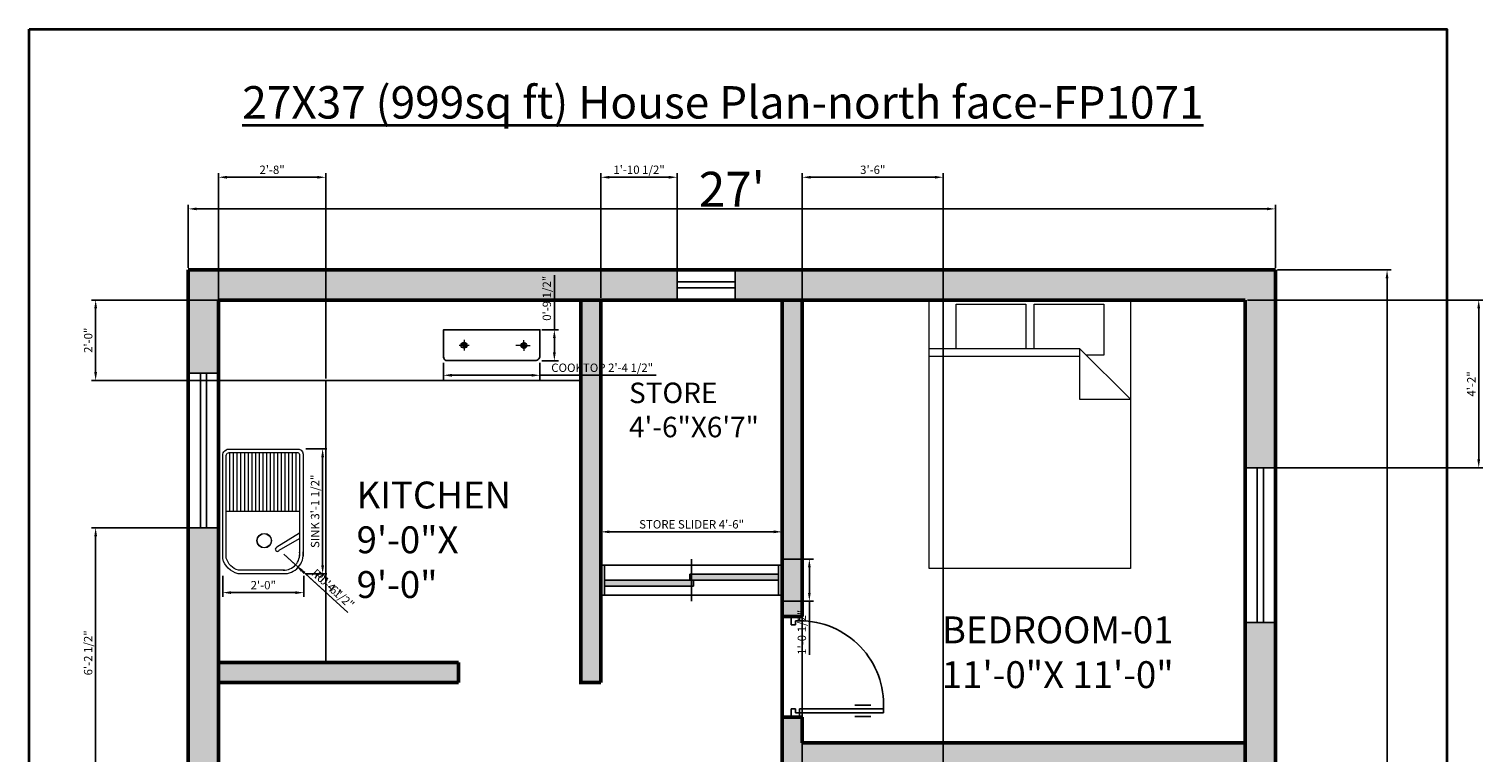
# Model space of a CAD drawing. Units: inches. Extents: x -36 to 398, y -51 to 516.
# Tile 3 of 3: x -36 to 398, y 300 to 516. Entities that reach past the tile are written whole.
import ezdxf

# ---------------------------------------------------------------- set-up
doc = ezdxf.new("R2010")
doc.units = ezdxf.units.IN
doc.header["$PDMODE"] = 34
for name, color, linetype, lineweight in [('A-ANNO-DIMS', 2, 'Continuous', 18), ('A-ANNO-TTLB', 7, 'Continuous', 35), ('A-AREA-IDEN', 7, 'Continuous', 25), ('A-DOOR', 170, 'Continuous', 25), ('A-EQPM', 8, 'Continuous', 18), ('A-FLOR-CASE', 7, 'Continuous', 25), ('A-FLOR-FIXT', 8, 'Continuous', 18), ('A-FURN', 8, 'Continuous', 18), ('A-GLAZ-PATT', 7, 'Continuous', 13), ('WALL', 7, 'Continuous', 50), ('WINDOW', 5, 'Continuous', 25)]:
    doc.layers.add(name, color=color, linetype=linetype, lineweight=lineweight)
doc.layers.add('A-WALL-PATT', color=251, linetype='Continuous', lineweight=13, true_color=0x636466)
doc.layers.add('dimensions', color=7, linetype='Continuous')
doc.styles.get("Standard").update_dxf_attribs({"font": 'arial.ttf'})
doc.dimstyles.new('ISO-25', dxfattribs={"dimtxt": 2.5, "dimasz": 2.5, "dimexe": 1.25, "dimexo": 0.625, "dimtad": 1, "dimdec": 1, "dimlunit": 3, "dimtxsty": 'Standard', "dimcen": 2.5, "dimadec": 0, "dimazin": 0, "dimtfac": 1, "dimtdec": 1, "dimtmove": 0, "dimatfit": 3, "dimfxl": 1, "dimarcsym": 0})

# ---------------------------------------------------------------- blocks, each defined once
blk = doc.blocks.new('WD_00_X1')
for p, q in [((-0.5, 0.5), (0.5, 0.5)), ((-0.48, 0.5), (-0.48, -0.5)), ((0.48, 0.5), (0.48, -0.5)), ((0.48, 0.1), (-0.48, 0.1)), ((0.48, -0.1), (-0.48, -0.1)), ((-0.5, -0.5), (0.5, -0.5))]:
    blk.add_line(p, q)
blk = doc.blocks.new('DR_UKF1')
for p, q in [((-0.458, 0.042), (-0.458, 0.875)), ((-0.458, 0.875), (-0.417, 0.875)), ((-0.417, 0.875), (-0.417, 0.042)), ((-0.494, 0.751), (-0.494, 0.59)), ((-0.381, 0.751), (-0.381, 0.59)), ((-0.5, -0.042), (-0.5, 0.042)), ((-0.5, 0.042), (-0.458, 0.042)), ((-0.417, 0.042), (-0.458, 0.042)), ((-0.458, 0.042), (-0.458, 0)), ((-0.458, 0), (-0.417, 0)), ((-0.417, 0), (-0.417, -0.042)), ((0.417, 0), (0.417, -0.042)), ((0.458, 0), (0.417, 0)), ((0.458, 0.042), (0.458, 0)), ((0.5, 0.042), (0.458, 0.042)), ((0.5, -0.042), (0.5, 0.042)), ((-0.417, -0.042), (-0.5, -0.042)), ((-0.5, -0.042), (-0.5, -0.042)), ((0.417, -0.042), (0.5, -0.042)), ((0.5, -0.042), (0.5, -0.042))]:
    blk.add_line(p, q)
blk.add_arc((-0.375, 0.043), 0.833, 359.9283, 92.866)
blk = doc.blocks.new('SINK')
for p, q in [((2.41, 0.46), (2.41, -20.67)), ((3.73, 0.46), (3.73, -20.67)), ((5.05, 0.46), (5.05, -20.67)), ((6.38, 0.46), (6.38, -20.67)), ((7.7, 0.46), (7.7, -20.67)), ((9.03, 0.46), (9.03, -20.67)), ((10.35, 0.46), (10.35, -20.67)), ((11.67, 0.46), (11.67, -20.67)), ((13, 0.46), (13, -20.67)), ((14.32, 0.46), (14.32, -20.67)), ((15.64, 0.46), (15.64, -20.67)), ((16.97, 0.46), (16.97, -20.67)), ((18.29, 0.46), (18.29, -20.67)), ((19.62, 0.46), (19.62, -20.67)), ((20.94, 0.46), (20.94, -20.67)), ((22.26, 0.46), (22.26, -20.67)), ((23.59, 0.46), (23.59, -20.67)), ((24.91, 0.46), (24.91, -20.67)), ((26.24, 0.46), (26.24, -20.67)), ((1.2, -20.67), (27.56, -20.67)), ((27.56, -28.49), (19.38, -33.59)), ((20.23, -34.64), (27.56, -30.49))]:
    blk.add_line(p, q)
for points in [[(22.1, -43.09), (5.43, -43.09, -0.278946), (-0.08, -37.68), (-0.08, -0.62, -0.442838), (2.54, 1.74, -0.442838)], [(22.1, -41.81), (5.59, -41.81, -0.266071), (1.2, -37.51), (1.2, -0.62, -0.442099), (2.41, 0.46)], [(2.18, 1.74), (26.61, 1.74, -0.390462), (28.84, -0.06), (28.84, -20.67)], [(2.18, 0.46), (26.66, 0.46, -0.376515), (27.56, -0.18), (27.56, -20.67)]]:
    blk.add_lwpolyline(points, format="xyb")
for points in [[(27.56, -0.18), (27.56, -36.84)], [(28.84, -0.18), (28.84, -36.84)]]:
    blk.add_lwpolyline(points)
for radius in [2.63, 2.53]:
    blk.add_circle((14.84, -31.22), radius)
for centre, radius, start, end in [((19.56, -34.32), 0.748, 103.6237, 334.3933), ((21.9, -36.1), 6.99, 267.9726, 7.4622), ((21.9, -36.1), 5.71, 267.9726, 7.4622)]:
    blk.add_arc(centre, radius, start, end)
blk = doc.blocks.new('WD_00_X2')
for p, q in [((0, 0.7), (0, -0.7)), ((-0.5, 0.5), (0.5, 0.5)), ((-0.48, 0.5), (-0.48, -0.5)), ((0.48, 0.5), (0.48, -0.5)), ((0.01, 0.2), (-0.48, 0.2)), ((0.01, 0.2), (0.01, 0)), ((0.48, 0), (-0.48, 0)), ((-0.01, 0), (-0.01, -0.2)), ((0.48, -0.2), (-0.01, -0.2)), ((-0.5, -0.5), (0.5, -0.5))]:
    blk.add_line(p, q)
blk = doc.blocks.new('GAS STOVE')
at = {"layer": 'dimensions'}
for points in [[(0.01, -8.39), (0, -8.07), (0, 0), (28.69, 0), (28.69, -7.85)], [(26.99, -9.22), (0.89, -9.22)]]:
    blk.add_lwpolyline(points, dxfattribs=at)
for centre, radius, start, end in [((0.99, -8.22), 1, 171.6035, 275.6391), ((27.21, -7.75), 1.48, 261.2373, 356.1184)]:
    blk.add_arc(centre, radius, start, end, dxfattribs=at)
for p in [(6.09, -4.63), (23.92, -4.73)]:
    blk.add_point(p, dxfattribs=at)
blk = doc.blocks.new('new block')
for p, q in [((6.13, -3.04), (6.13, -6.22)), ((23.92, -4.73), (23.92, -3.08)), ((4.65, -4.66), (7.63, -4.66)), ((23.92, -4.73), (21.5, -4.73)), ((23.92, -4.73), (25.8, -4.73)), ((23.92, -4.73), (23.92, -6.28))]:
    blk.add_line(p, q)
for centre, radius in [((6.09, -4.63), 0.897), ((23.92, -4.73), 0.857)]:
    blk.add_circle(centre, radius)
blk.add_blockref('GAS STOVE', (0, 0))
blk = doc.blocks.new('Bed - Queen')
for p, q in [((0, -80.00003), (0, 0)), ((0, 0), (59.99999, 0)), ((59.99999, 0), (59.99999, -80.00003)), ((7.99999, -1.2), (28.79998, -1.2)), ((7.99999, -14.4), (7.99999, -1.2)), ((28.79998, -1.2), (28.79998, -14.4)), ((31.19999, -1.2), (51.99999, -1.2)), ((31.19999, -14.4), (31.19999, -1.2)), ((51.99999, -1.2), (51.99999, -16.4)), ((0, -14.4), (44.8, -14.4)), ((44.8, -16.8), (0, -16.8)), ((59.99999, -29.6), (44.8, -14.4)), ((44.8, -14.4), (44.8, -29.6)), ((51.99999, -16.4), (46.79936, -16.4)), ((44.8, -29.6), (59.99999, -29.6)), ((59.99999, -80.00003), (0, -80.00003))]:
    blk.add_line(p, q)
blk = doc.blocks.new('*D15')
at = {"layer": 'A-ANNO-DIMS', "color": 0, "lineweight": -2, "transparency": 16777216}
for p, q in [((11.71, 444.6), (11.71, 463.4)), ((14.21, 462.15), (333.21, 462.15)), ((335.71, 444.6), (335.71, 463.4))]:
    blk.add_line(p, q, dxfattribs=at)
at = {"layer": 'A-ANNO-DIMS', "color": 0, "transparency": 16777216}
for points in [[(14.21, 462.57), (14.21, 461.73), (11.71, 462.15)], [(333.21, 462.57), (333.21, 461.73), (335.71, 462.15)]]:
    blk.add_solid(points, dxfattribs=at)
at = {"layer": 'Defpoints', "color": 0, "transparency": 16777216}
for p in [(335.71, 462.15), (11.71, 443.98), (335.71, 443.98)]:
    blk.add_point(p, dxfattribs=at)
at = {"layer": 'A-ANNO-DIMS', "color": 0, "transparency": 16777216, "insert": (173.71, 468), "char_height": 2.5, "attachment_point": 5}
blk.add_mtext("{\\H4.16x;27'}", dxfattribs=at)
blk = doc.blocks.new('*D16')
at = {"layer": 'A-ANNO-DIMS', "color": 0, "lineweight": -2, "transparency": 16777216}
for p, q in [((336.34, 443.98), (370.23, 443.98)), ((368.98, 441.48), (368.98, 2.48)), ((336.34, -0.02), (370.23, -0.02))]:
    blk.add_line(p, q, dxfattribs=at)
at = {"layer": 'A-ANNO-DIMS', "color": 0, "transparency": 16777216}
for points in [[(368.56, 441.48), (369.39, 441.48), (368.98, 443.98)], [(368.56, 2.48), (369.39, 2.48), (368.98, -0.02)]]:
    blk.add_solid(points, dxfattribs=at)
at = {"layer": 'Defpoints', "color": 0, "transparency": 16777216}
for p in [(335.71, 443.98), (335.71, -0.02), (368.98, -0.02)]:
    blk.add_point(p, dxfattribs=at)
at = {"layer": 'A-ANNO-DIMS', "color": 0, "transparency": 16777216, "insert": (363.04, 221.98), "char_height": 2.5, "attachment_point": 5, "rotation": 90}
blk.add_mtext("{\\H4.16x;37'}", dxfattribs=at)
blk = doc.blocks.new('*D28')
at = {"layer": 'A-ANNO-DIMS', "color": 0, "lineweight": -2, "transparency": 16777216}
for p, q in [((46.79, 390.64), (53, 390.64)), ((51.75, 355.86), (51.75, 388.14)), ((46.79, 353.36), (53, 353.36))]:
    blk.add_line(p, q, dxfattribs=at)
at = {"layer": 'A-ANNO-DIMS', "color": 0, "transparency": 16777216}
for points in [[(51.34, 388.14), (52.17, 388.14), (51.75, 390.64)], [(51.34, 355.86), (52.17, 355.86), (51.75, 353.36)]]:
    blk.add_solid(points, dxfattribs=at)
at = {"layer": 'Defpoints', "color": 0, "transparency": 16777216}
for p in [(46.16, 390.64), (51.75, 390.64), (46.16, 353.36)]:
    blk.add_point(p, dxfattribs=at)
at = {"layer": 'A-ANNO-DIMS', "color": 0, "transparency": 16777216, "insert": (49.83, 372), "char_height": 2.5, "attachment_point": 5, "rotation": 90}
blk.add_mtext('SINK 3\'-1 1/2"', dxfattribs=at)
blk = doc.blocks.new('*D29')
at = {"layer": 'A-ANNO-DIMS', "color": 0, "lineweight": -2, "transparency": 16777216}
for p, q in [((21.97, 352.73), (21.97, 346.51)), ((46.16, 352.73), (46.16, 346.51)), ((24.47, 347.76), (43.66, 347.76))]:
    blk.add_line(p, q, dxfattribs=at)
at = {"layer": 'A-ANNO-DIMS', "color": 0, "transparency": 16777216}
for points in [[(24.47, 348.18), (24.47, 347.35), (21.97, 347.76)], [(43.66, 348.18), (43.66, 347.35), (46.16, 347.76)]]:
    blk.add_solid(points, dxfattribs=at)
at = {"layer": 'Defpoints', "color": 0, "transparency": 16777216}
for p in [(21.97, 353.36), (46.16, 353.36), (46.16, 347.76)]:
    blk.add_point(p, dxfattribs=at)
at = {"layer": 'A-ANNO-DIMS', "color": 0, "transparency": 16777216, "insert": (34.07, 349.66), "char_height": 2.5, "attachment_point": 5}
blk.add_mtext('2\'-0"', dxfattribs=at)
blk = doc.blocks.new('*D30')
at = {"layer": 'A-ANNO-DIMS', "color": 0, "lineweight": -2, "transparency": 16777216}
for p, q in [((134.71, 358.41), (134.71, 367.13)), ((137.21, 365.88), (186.21, 365.88)), ((188.71, 358.41), (188.71, 367.13))]:
    blk.add_line(p, q, dxfattribs=at)
at = {"layer": 'A-ANNO-DIMS', "color": 0, "transparency": 16777216}
for points in [[(137.21, 366.3), (137.21, 365.47), (134.71, 365.88)], [(186.21, 366.3), (186.21, 365.47), (188.71, 365.88)]]:
    blk.add_solid(points, dxfattribs=at)
at = {"layer": 'Defpoints', "color": 0, "transparency": 16777216}
for p in [(188.71, 365.88), (134.71, 357.78), (188.71, 357.78)]:
    blk.add_point(p, dxfattribs=at)
at = {"layer": 'A-ANNO-DIMS', "color": 0, "transparency": 16777216, "insert": (161.71, 367.8), "char_height": 2.5, "attachment_point": 5}
blk.add_mtext('STORE SLIDER 4\'-6"', dxfattribs=at)
blk = doc.blocks.new('*D31')
at = {"layer": 'A-ANNO-DIMS', "color": 0, "lineweight": -2, "transparency": 16777216}
for p, q in [((189.34, 357.78), (198.06, 357.78)), ((196.81, 355.28), (196.81, 347.68)), ((189.34, 345.18), (198.06, 345.18)), ((196.81, 345.18), (196.81, 329.2))]:
    blk.add_line(p, q, dxfattribs=at)
at = {"layer": 'A-ANNO-DIMS', "color": 0, "transparency": 16777216}
for points in [[(196.4, 355.28), (197.23, 355.28), (196.81, 357.78)], [(196.4, 347.68), (197.23, 347.68), (196.81, 345.18)]]:
    blk.add_solid(points, dxfattribs=at)
at = {"layer": 'Defpoints', "color": 0, "transparency": 16777216}
for p in [(188.71, 357.78), (188.71, 345.18), (196.81, 345.18)]:
    blk.add_point(p, dxfattribs=at)
at = {"layer": 'A-ANNO-DIMS', "color": 0, "transparency": 16777216, "insert": (194.9, 335.94), "char_height": 2.5, "attachment_point": 5, "rotation": 90}
blk.add_mtext('1\'-0 1/2"', dxfattribs=at)
blk = doc.blocks.new('*D32')
at = {"layer": 'A-ANNO-DIMS', "color": 0, "lineweight": -2, "transparency": 16777216}
for p, q in [((87.77, 416.23), (87.77, 411.3)), ((116.51, 416.23), (116.51, 411.3)), ((90.27, 412.55), (114.01, 412.55)), ((116.51, 412.55), (151.13, 412.55))]:
    blk.add_line(p, q, dxfattribs=at)
at = {"layer": 'A-ANNO-DIMS', "color": 0, "transparency": 16777216}
for points in [[(90.27, 412.97), (90.27, 412.13), (87.77, 412.55)], [(114.01, 412.97), (114.01, 412.13), (116.51, 412.55)]]:
    blk.add_solid(points, dxfattribs=at)
at = {"layer": 'Defpoints', "color": 0, "transparency": 16777216}
for p in [(87.77, 416.86), (116.51, 416.86), (116.51, 412.55)]:
    blk.add_point(p, dxfattribs=at)
at = {"layer": 'A-ANNO-DIMS', "color": 0, "transparency": 16777216, "insert": (135.07, 414.47), "char_height": 2.5, "attachment_point": 5}
blk.add_mtext('COOKTOP 2\'-4 1/2"', dxfattribs=at)
blk = doc.blocks.new('*D33')
at = {"layer": 'A-ANNO-DIMS', "color": 0, "lineweight": -2, "transparency": 16777216}
for p, q in [((120.82, 426.14), (120.82, 442.36)), ((117.13, 426.14), (122.07, 426.14)), ((120.82, 419.36), (120.82, 423.64)), ((117.13, 416.86), (122.07, 416.86))]:
    blk.add_line(p, q, dxfattribs=at)
at = {"layer": 'A-ANNO-DIMS', "color": 0, "transparency": 16777216}
for points in [[(120.4, 423.64), (121.23, 423.64), (120.82, 426.14)], [(120.4, 419.36), (121.23, 419.36), (120.82, 416.86)]]:
    blk.add_solid(points, dxfattribs=at)
at = {"layer": 'Defpoints', "color": 0, "transparency": 16777216}
for p in [(116.51, 426.14), (120.82, 426.14), (116.51, 416.86)]:
    blk.add_point(p, dxfattribs=at)
at = {"layer": 'A-ANNO-DIMS', "color": 0, "transparency": 16777216, "insert": (118.9, 435.5), "char_height": 2.5, "attachment_point": 5, "rotation": 90}
blk.add_mtext('0\'-9 1/2"', dxfattribs=at)
blk = doc.blocks.new('*D39')
at = {"layer": 'A-ANNO-DIMS', "color": 0, "lineweight": -2, "transparency": 16777216}
for p, q in [((11.09, 367.07), (-17.14, 367.07)), ((-15.89, 295.04), (-15.89, 364.57)), ((11.09, 292.54), (-17.14, 292.54))]:
    blk.add_line(p, q, dxfattribs=at)
at = {"layer": 'A-ANNO-DIMS', "color": 0, "transparency": 16777216}
for points in [[(-16.3, 364.57), (-15.47, 364.57), (-15.89, 367.07)], [(-16.3, 295.04), (-15.47, 295.04), (-15.89, 292.54)]]:
    blk.add_solid(points, dxfattribs=at)
at = {"layer": 'Defpoints', "color": 0, "transparency": 16777216}
for p in [(-15.89, 367.07), (11.71, 367.07), (11.71, 292.54)]:
    blk.add_point(p, dxfattribs=at)
at = {"layer": 'A-ANNO-DIMS', "color": 0, "transparency": 16777216, "insert": (-17.8, 329.81), "char_height": 2.5, "attachment_point": 5, "rotation": 90}
blk.add_mtext('6\'-2 1/2"', dxfattribs=at)
blk = doc.blocks.new('*D40')
at = {"layer": 'A-ANNO-DIMS', "color": 0, "lineweight": -2, "transparency": 16777216}
for p, q in [((134.71, 435.6), (134.71, 472.83)), ((157.41, 435.6), (157.41, 472.83)), ((137.21, 471.58), (154.91, 471.58))]:
    blk.add_line(p, q, dxfattribs=at)
at = {"layer": 'A-ANNO-DIMS', "color": 0, "transparency": 16777216}
for points in [[(137.21, 471.99), (137.21, 471.16), (134.71, 471.58)], [(154.91, 471.99), (154.91, 471.16), (157.41, 471.58)]]:
    blk.add_solid(points, dxfattribs=at)
at = {"layer": 'Defpoints', "color": 0, "transparency": 16777216}
for p in [(157.41, 471.58), (134.71, 434.98), (157.41, 434.98)]:
    blk.add_point(p, dxfattribs=at)
at = {"layer": 'A-ANNO-DIMS', "color": 0, "transparency": 16777216, "insert": (146.06, 473.49), "char_height": 2.5, "attachment_point": 5}
blk.add_mtext('1\'-10 1/2"', dxfattribs=at)
blk = doc.blocks.new('*D41')
at = {"layer": 'A-ANNO-DIMS', "color": 0, "lineweight": -2, "transparency": 16777216}
for p, q in [((327.34, 434.98), (397.55, 434.98)), ((396.3, 432.48), (396.3, 387.47)), ((327.34, 384.97), (397.55, 384.97))]:
    blk.add_line(p, q, dxfattribs=at)
at = {"layer": 'A-ANNO-DIMS', "color": 0, "transparency": 16777216}
for points in [[(395.88, 432.48), (396.71, 432.48), (396.3, 434.98)], [(395.88, 387.47), (396.71, 387.47), (396.3, 384.97)]]:
    blk.add_solid(points, dxfattribs=at)
at = {"layer": 'Defpoints', "color": 0, "transparency": 16777216}
for p in [(326.71, 434.98), (326.71, 384.97), (396.3, 384.97)]:
    blk.add_point(p, dxfattribs=at)
at = {"layer": 'A-ANNO-DIMS', "color": 0, "transparency": 16777216, "insert": (394.42, 409.97), "char_height": 2.5, "attachment_point": 5, "rotation": 90}
blk.add_mtext('4\'-2"', dxfattribs=at)
blk = doc.blocks.new('*D45')
at = {"layer": 'A-ANNO-DIMS', "color": 0, "lineweight": -2, "transparency": 16777216}
for p, q in [((20.71, 413.78), (20.71, 472.83)), ((52.67, 411.6), (52.67, 472.83)), ((23.21, 471.58), (50.17, 471.58))]:
    blk.add_line(p, q, dxfattribs=at)
at = {"layer": 'A-ANNO-DIMS', "color": 0, "transparency": 16777216}
for points in [[(23.21, 471.99), (23.21, 471.16), (20.71, 471.58)], [(50.17, 471.99), (50.17, 471.16), (52.67, 471.58)]]:
    blk.add_solid(points, dxfattribs=at)
at = {"layer": 'Defpoints', "color": 0, "transparency": 16777216}
for p in [(52.67, 471.58), (20.71, 413.15), (52.67, 410.98)]:
    blk.add_point(p, dxfattribs=at)
at = {"layer": 'A-ANNO-DIMS', "color": 0, "transparency": 16777216, "insert": (36.69, 473.48), "char_height": 2.5, "attachment_point": 5}
blk.add_mtext('2\'-8"', dxfattribs=at)
blk = doc.blocks.new('*D46')
at = {"layer": 'A-ANNO-DIMS', "color": 0, "lineweight": -2, "transparency": 16777216}
for p, q in [((128.09, 434.98), (-17.14, 434.98)), ((-15.89, 413.48), (-15.89, 432.48)), ((128.09, 410.98), (-17.14, 410.98))]:
    blk.add_line(p, q, dxfattribs=at)
at = {"layer": 'A-ANNO-DIMS', "color": 0, "transparency": 16777216}
for points in [[(-16.3, 432.48), (-15.47, 432.48), (-15.89, 434.98)], [(-16.3, 413.48), (-15.47, 413.48), (-15.89, 410.98)]]:
    blk.add_solid(points, dxfattribs=at)
at = {"layer": 'Defpoints', "color": 0, "transparency": 16777216}
for p in [(-15.89, 434.98), (128.71, 434.98), (128.71, 410.98)]:
    blk.add_point(p, dxfattribs=at)
at = {"layer": 'A-ANNO-DIMS', "color": 0, "transparency": 16777216, "insert": (-17.79, 422.98), "char_height": 2.5, "attachment_point": 5, "rotation": 90}
blk.add_mtext('2\'-0"', dxfattribs=at)
blk = doc.blocks.new('*D50')
at = {"layer": 'A-ANNO-DIMS', "color": 0, "lineweight": -2, "transparency": 16777216}
for p, q in [((194.71, 248.83), (194.71, 472.83)), ((236.71, 277.21), (236.71, 472.83)), ((197.21, 471.58), (234.21, 471.58))]:
    blk.add_line(p, q, dxfattribs=at)
at = {"layer": 'A-ANNO-DIMS', "color": 0, "transparency": 16777216}
for points in [[(197.21, 471.99), (197.21, 471.16), (194.71, 471.58)], [(234.21, 471.99), (234.21, 471.16), (236.71, 471.58)]]:
    blk.add_solid(points, dxfattribs=at)
at = {"layer": 'Defpoints', "color": 0, "transparency": 16777216}
for p in [(236.71, 471.58), (236.71, 276.58), (194.71, 248.21)]:
    blk.add_point(p, dxfattribs=at)
at = {"layer": 'A-ANNO-DIMS', "color": 0, "transparency": 16777216, "insert": (215.71, 473.48), "char_height": 2.5, "attachment_point": 5}
blk.add_mtext('3\'-6"', dxfattribs=at)
blk = doc.blocks.new('*D53')
at = {"layer": 'A-ANNO-DIMS', "color": 0, "lineweight": -2, "transparency": 16777216}
for p, q in [((40.19, 359.21), (44.48, 355.31)), ((55.79, 345.02), (46.33, 353.63))]:
    blk.add_line(p, q, dxfattribs=at)
at = {"layer": 'A-ANNO-DIMS', "color": 0, "transparency": 16777216}
blk.add_solid([(46.61, 353.94), (46.05, 353.32), (44.48, 355.31)], dxfattribs=at)
at = {"layer": 'Defpoints', "color": 0, "transparency": 16777216}
for p in [(40.19, 359.21), (44.48, 355.31)]:
    blk.add_point(p, dxfattribs=at)
at = {"layer": 'A-ANNO-DIMS', "color": 0, "transparency": 16777216, "insert": (53.26, 349.89), "char_height": 2.5, "attachment_point": 5, "rotation": 317.7157}
blk.add_mtext('R0\'-6"', dxfattribs=at)
blk = doc.blocks.new('*D54')
at = {"layer": 'A-ANNO-DIMS', "color": 0, "lineweight": -2, "transparency": 16777216}
for p, q in [((40.19, 359.21), (43.69, 356.02)), ((59.31, 341.82), (45.54, 354.34))]:
    blk.add_line(p, q, dxfattribs=at)
at = {"layer": 'A-ANNO-DIMS', "color": 0, "transparency": 16777216}
blk.add_solid([(45.82, 354.65), (45.26, 354.03), (43.69, 356.02)], dxfattribs=at)
at = {"layer": 'Defpoints', "color": 0, "transparency": 16777216}
for p in [(40.19, 359.21), (43.69, 356.02)]:
    blk.add_point(p, dxfattribs=at)
at = {"layer": 'A-ANNO-DIMS', "color": 0, "transparency": 16777216, "insert": (54.64, 348.66), "char_height": 2.5, "attachment_point": 5, "rotation": 317.7166}
blk.add_mtext('R0\'-4 1/2"', dxfattribs=at)

msp = doc.modelspace()

# ---------------------------------------------------------------- hatches: boundary and pattern name
at = {"layer": 'A-GLAZ-PATT'}
h = msp.add_hatch(color=256, dxfattribs=at)
h.dxf.hatch_style = 1
h.paths.add_polyline_path([(187.63, 351.48), (187.63, 353.28), (161.71, 353.28), (161.71, 351.48)])
h.paths.add_polyline_path([(135.79, 351.48), (135.79, 349.68), (161.71, 349.68), (161.71, 351.48)])
at = {"layer": 'A-WALL-PATT'}
h = msp.add_hatch(color=256, dxfattribs=at)
h.dxf.hatch_style = 1
h.paths.add_polyline_path([(335.71, 155.4), (326.71, 155.4), (326.71, 154.44), (326.71, 50.65), (335.71, 50.65), (335.71, 51.01)])
h.paths.add_polyline_path([(335.71, 257.33), (326.71, 257.33), (326.71, 256.97), (326.71, 201.48), (335.71, 201.48), (335.71, 202.44)])
h.paths.add_polyline_path([(335.71, 33.37), (326.71, 33.37), (326.71, 33.01), (326.71, 8.98), (200.71, 8.98), (148.47, 8.98), (148.47, -0.02), (335.71, -0.02)])
h.paths.add_polyline_path([(118.44, 5.24), (118.46, 8.98), (92.19, 8.98), (92.19, -0.02), (93.15, -0.02), (118.46, -0.02), (118.46, 2.74), (118.44, 2.74)])
h.paths.add_polyline_path([(20.71, 85.44), (11.71, 85.44), (11.71, 84.48), (11.71, -0.02), (46.11, -0.02), (46.11, 8.98), (45.15, 8.98), (20.71, 8.98)])
h.paths.add_polyline_path([(20.71, 246.46), (11.71, 246.46), (11.71, 245.5), (11.71, 131.52), (20.71, 131.52), (20.71, 132.48)])
h.paths.add_polyline_path([(152.93, 182.98), (20.71, 182.98), (20.71, 176.98), (152.93, 176.98)])
h.paths.add_polyline_path([(188.71, 182.98), (182.93, 182.98), (182.93, 176.98), (188.71, 176.98)])
h.paths.add_polyline_path([(194.71, 224.98), (199.29, 224.98), (199.29, 230.98), (188.71, 230.98), (188.71, 79.98), (210.71, 79.98), (210.71, 80.98), (326.71, 80.98), (326.71, 85.98), (194.71, 85.98)])
h.paths.add_polyline_path([(326.71, 230.98), (229.41, 230.98), (229.41, 224.98), (326.71, 224.98)], flags=0)
h.paths.add_polyline_path([(242.71, 276.58), (236.71, 276.58), (236.71, 230.98), (242.71, 230.98)])
h.paths.add_polyline_path([(326.71, 302.98), (194.71, 302.98), (194.71, 310.64), (188.71, 310.64), (188.71, 296.98), (326.71, 296.98)])
h.paths.add_polyline_path([(242.71, 296.98), (236.71, 296.98), (236.71, 294.58), (242.71, 294.58)])
h.paths.add_polyline_path([(194.71, 434.98), (188.71, 434.98), (188.71, 340.61), (191.4, 340.61), (191.4, 340.64), (193.9, 340.64), (194.71, 340.61)])
h.paths.add_polyline_path([(335.71, 443.98), (174.69, 443.98), (174.69, 434.98), (175.05, 434.98), (326.71, 434.98), (326.71, 384.97), (335.71, 384.97), (335.71, 385.93)])
h.paths.add_polyline_path([(335.71, 338.89), (326.71, 338.89), (326.71, 337.93), (326.71, 274.61), (335.71, 274.61), (335.71, 274.97)])
h.paths.add_polyline_path([(157.41, 443.98), (157.05, 443.98), (11.71, 443.98), (11.71, 413.15), (20.71, 413.15), (20.71, 414.11), (20.71, 434.98), (157.41, 434.98)])
h.paths.add_polyline_path([(20.71, 367.07), (11.71, 367.07), (11.71, 366.11), (11.71, 292.54), (20.71, 292.54), (20.71, 293.5)])
h = msp.add_hatch(color=256, dxfattribs=at)
h.dxf.hatch_style = 1
h.paths.add_polyline_path([(20.71, 326.98), (20.71, 320.98), (92.29, 320.98), (92.29, 326.98)])
h.paths.add_polyline_path([(128.71, 320.98), (134.71, 320.98), (134.71, 434.98), (128.71, 434.98)])

# ---------------------------------------------------------------- linework, layer by layer
at = {"layer": 'A-ANNO-TTLB'}
msp.add_lwpolyline([(-35.73, 515.75), (386.76, 515.75), (386.76, -51.27), (-35.73, -51.27)], close=True, dxfattribs=at)
at = {"layer": 'A-FLOR-CASE'}
for p, q in [((128.71, 410.98), (52.67, 410.98)), ((52.67, 410.98), (52.67, 326.98))]:
    msp.add_line(p, q, dxfattribs=at)
at = {"layer": 'WALL'}
for p, q in [((11.71, -0.02), (11.71, 443.98)), ((11.71, 443.98), (335.71, 443.98)), ((335.71, -0.02), (335.71, 443.98)), ((20.71, 434.98), (326.71, 434.98)), ((20.71, 434.98), (20.71, 8.98)), ((128.71, 320.98), (128.71, 434.98)), ((134.71, 320.98), (134.71, 434.98)), ((188.71, 296.98), (188.71, 434.98)), ((194.71, 340.61), (194.71, 434.98)), ((326.71, 8.98), (326.71, 434.98)), ((194.71, 340.61), (188.71, 340.61)), ((20.71, 326.98), (92.29, 326.98)), ((92.29, 320.98), (92.29, 326.98)), ((20.71, 320.98), (92.29, 320.98)), ((128.21, 320.98), (134.71, 320.98)), ((188.71, 310.64), (194.71, 310.64)), ((194.71, 302.98), (194.71, 310.64)), ((194.71, 302.98), (326.71, 302.98))]:
    msp.add_line(p, q, dxfattribs=at)

# ---------------------------------------------------------------- block references
at = {"layer": 'A-DOOR', "xscale": -30, "yscale": 30, "zscale": 30, "rotation": 270.0000000000237}
msp.add_blockref('DR_UKF1', (192.65, 325.64), dxfattribs=at)
at = {"layer": 'A-EQPM'}
msp.add_blockref('new block', (87.82, 426.14), dxfattribs=at)
at = {"layer": 'A-FLOR-FIXT', "xscale": 0.8289137605783039, "yscale": 0.8289137605783039, "zscale": 0.8289137605783039}
msp.add_blockref('SINK', (22.04, 389.13), dxfattribs=at)
at = {"layer": 'A-FURN'}
msp.add_blockref('Bed - Queen', (232.56, 434.98), dxfattribs=at)
at = {"layer": 'WINDOW', "xscale": 18, "yscale": 9, "zscale": 18}
msp.add_blockref('WD_00_X1', (166.05, 439.48), dxfattribs=at)
at = {"layer": 'WINDOW', "yscale": 9}
for name, p, xscale, zscale, rotation in [('WD_00_X1', (16.21, 390.11), 48, 48, 89.99999999999999), ('WD_00_X1', (331.21, 361.93), 48, 48, 89.99999999999999), ('WD_00_X2', (161.71, 351.48), -54, 54, 180)]:
    msp.add_blockref(name, p, dxfattribs=dict(at, xscale=xscale, zscale=zscale, rotation=rotation))

# ---------------------------------------------------------------- texts
at = {"layer": 'A-ANNO-TTLB', "insert": (27.79, 498.74), "char_height": 9.6617, "attachment_point": 1}
msp.add_mtext_dynamic_manual_height_columns('{\\fArial|b1|i0|c0|p34;\\L27X37 (999sq ft) House Plan-north face-FP1071}', width=305.8474, gutter_width=48.31, heights=[0], dxfattribs=at)
at = {"layer": 'A-AREA-IDEN', "attachment_point": 1}
for s, width, gutter_width, insert, char_height in [('STORE \\P4\'-6"X6\'7"', 43.6398, 30.54, (143.07, 410.36), 6.108), ('KITCHEN\\P9\'-0"X 9\'-0"', 56.1888, 40.03, (61.87, 380.86), 8.0065), ('BEDROOM-01\\P11\'-0"X 11\'-0"', 96.1834, 40.03, (236.29, 340.66), 8.0065)]:
    msp.add_mtext_dynamic_manual_height_columns(s, width=width, gutter_width=gutter_width, heights=[0], dxfattribs=dict(at, insert=insert, char_height=char_height))

# ---------------------------------------------------------------- dimensions: what is measured, and where the dimension line sits
at = {"layer": 'A-ANNO-DIMS'}
for base, p1, p2, picture, middle in [((157.41, 471.58), (134.71, 434.98), (157.41, 434.98), '*D40', (146.06, 473.49)), ((52.67, 471.58), (20.71, 413.15), (52.67, 410.98), '*D45', (36.69, 473.48)), ((236.71, 471.58), (194.71, 248.21), (236.71, 276.58), '*D50', (215.71, 473.48)), ((46.16, 347.76), (21.97, 353.36), (46.16, 353.36), '*D29', (34.07, 349.66))]:
    dim = msp.add_linear_dim(base=base, p1=p1, p2=p2, dimstyle='ISO-25', override={"dimdec": 1, "dimlfac": 1, "dimrnd": 0, "dimzin": 1, "dimdsep": 46, "dimlunit": 4, "dimfrac": 2}, dxfattribs=at)
    dim.commit()
    dim.dimension.update_dxf_attribs({"geometry": picture, "text_midpoint": middle})
for base, p1, p2, text, override, picture, middle in [((335.71, 462.15), (11.71, 443.98), (335.71, 443.98), '{\\H4.16x;<>}', {"dimclrd": 0, "dimclre": 0, "dimclrt": 0}, '*D15', (173.71, 468)), ((116.51, 412.55), (87.77, 416.86), (116.51, 416.86), 'COOKTOP <>', {"dimdec": 1, "dimlfac": 1, "dimrnd": 0, "dimzin": 1, "dimdsep": 46, "dimlunit": 4, "dimfrac": 2}, '*D32', (135.07, 414.47)), ((188.71, 365.88), (134.71, 357.78), (188.71, 357.78), 'STORE SLIDER <>', {"dimdec": 1, "dimlfac": 1, "dimrnd": 0, "dimzin": 1, "dimdsep": 46, "dimlunit": 4, "dimfrac": 2}, '*D30', (161.71, 367.8))]:
    dim = msp.add_linear_dim(base=base, p1=p1, p2=p2, text=text, dimstyle='ISO-25', override=override, dxfattribs=at)
    dim.commit()
    dim.dimension.update_dxf_attribs({"geometry": picture, "text_midpoint": middle})
for base, p1, p2, angle, picture, middle in [((120.82, 426.14), (116.51, 416.86), (116.51, 426.14), 90, '*D33', (118.9, 435.5)), ((-15.89, 434.98), (128.71, 410.98), (128.71, 434.98), 90, '*D46', (-17.79, 422.98)), ((396.3, 384.97), (326.71, 434.98), (326.71, 384.97), 90, '*D41', (394.42, 409.97)), ((-15.89, 367.07), (11.71, 292.54), (11.71, 367.07), 90, '*D39', (-17.8, 329.81)), ((196.81, 345.18), (188.71, 357.78), (188.71, 345.18), 270, '*D31', (194.9, 335.94))]:
    dim = msp.add_linear_dim(base=base, p1=p1, p2=p2, angle=angle, dimstyle='ISO-25', override={"dimdec": 1, "dimlfac": 1, "dimrnd": 0, "dimzin": 1, "dimdsep": 46, "dimlunit": 4, "dimfrac": 2}, dxfattribs=at)
    dim.commit()
    dim.dimension.update_dxf_attribs({"geometry": picture, "text_midpoint": middle})
for base, p1, p2, text, override, picture, middle in [((368.98, -0.02), (335.71, 443.98), (335.71, -0.02), '{\\H4.16x;<>}', {"dimclrd": 0, "dimclre": 0, "dimclrt": 0}, '*D16', (363.04, 221.98)), ((51.75, 390.64), (46.16, 353.36), (46.16, 390.64), 'SINK <>', {"dimdec": 1, "dimlfac": 1, "dimrnd": 0, "dimzin": 1, "dimdsep": 46, "dimlunit": 4, "dimfrac": 2}, '*D28', (49.83, 372))]:
    dim = msp.add_linear_dim(base=base, p1=p1, p2=p2, angle=90, text=text, dimstyle='ISO-25', override=override, dxfattribs=at)
    dim.commit()
    dim.dimension.update_dxf_attribs({"geometry": picture, "text_midpoint": middle})
for mpoint, picture, middle in [((44.48, 355.31), '*D53', (53.26, 349.89)), ((43.69, 356.02), '*D54', (54.64, 348.66))]:
    dim = msp.add_radius_dim(center=(40.19, 359.21), mpoint=mpoint, dimstyle='ISO-25', override={"dimdec": 1, "dimlfac": 1, "dimrnd": 0, "dimzin": 1, "dimdsep": 46, "dimlunit": 4, "dimfrac": 2}, dxfattribs=at)
    dim.commit()
    dim.dimension.update_dxf_attribs({"geometry": picture, "text_midpoint": middle})

doc.saveas('drawing.dxf')
